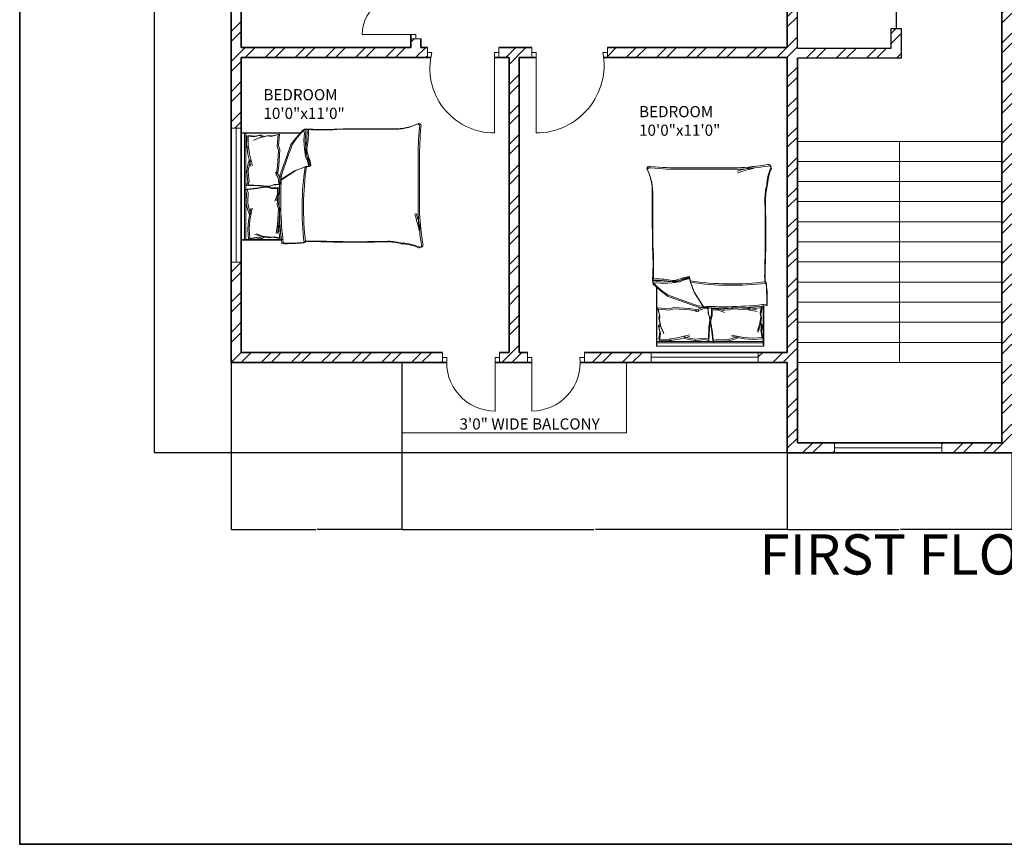
# Model space of a CAD drawing. Units: inches. Extents: x 2165 to 3042, y 1626 to 2968.
# Tile 1 of 11: x 2192 to 2633, y 1626 to 1996. Entities that reach past the tile are written whole.
import ezdxf

# ---------------------------------------------------------------- set-up
doc = ezdxf.new("R2010")
doc.units = ezdxf.units.IN
for name, color, linetype, lineweight in [('A-ANNO-DIMS', 2, 'Continuous', 18), ('A-ANNO-TEXT', 7, 'Continuous', 25), ('A-AREA-IDEN', 7, 'Continuous', 18), ('A-DOOR', 3, 'Continuous', 18), ('A-FLOR-BALC', 7, 'Continuous', 18), ('A-FLOR-EVTR', 7, 'Continuous', 25), ('A-FLOR-STRS', 7, 'Continuous', 18), ('A-FURN', 8, 'Continuous', 13), ('A-GLAZ', 4, 'Continuous', 18), ('A-WALL', 7, 'Continuous', 35), ('A-WALL-PATT', 252, 'Continuous', 13)]:
    doc.layers.add(name, color=color, linetype=linetype, lineweight=lineweight)
doc.styles.get("Standard").update_dxf_attribs({"font": 'arial.ttf'})
doc.dimstyles.get("Standard").update_dxf_attribs({"dimtxt": 0.18, "dimasz": 0.18, "dimexe": 0.18, "dimexo": 0.0625, "dimgap": 0.09, "dimtad": 0, "dimtih": 1, "dimtoh": 1, "dimdec": 4, "dimzin": 0, "dimdsep": 46, "dimtxsty": 'Standard', "dimcen": 0.09, "dimadec": 0, "dimazin": 0, "dimtfac": 1, "dimtdec": 4, "dimtofl": 0, "dimtmove": 0, "dimatfit": 3, "dimfxl": 1, "dimtolj": 1, "dimtzin": 0, "dimarcsym": 0})

# ---------------------------------------------------------------- blocks, each defined once
blk = doc.blocks.new('BED-DOUBLE')
for p, q in [((28.39, 53.1), (25.14, 49.39)), ((28.39, 53.1), (25.14, 49.39)), ((29.49, 52.95), (27.75, 52.87, 3.87)), ((29.49, 52.95), (27.75, 52.87, 3.87)), ((30.13, 53.18), (28.39, 53.1, 3.87)), ((30.13, 53.18), (28.39, 53.1, 3.87)), ((29, 51.56), (28.39, 53.1)), ((29, 51.56), (28.39, 53.1)), ((0, 51.27), (0, 51.49)), ((0, 51.49), (0.64, 51.49)), ((0, 51.27), (26.61, 51.27)), ((0, 51.27), (26.61, 51.27)), ((0, 51.27), (0, 3.48)), ((0.64, 51.49), (27.25, 51.49)), ((0.64, 51.49), (27.25, 51.49)), ((1.53, 3.48), (1.53, 51.27)), ((1.53, 3.47), (1.53, 51.27)), ((2.17, 3.7), (2.17, 51.49)), ((2.17, 3.7), (2.17, 51.49)), ((2.56, 50.11), (2.46, 44.71)), ((2.56, 50.11), (2.46, 44.71)), ((2.56, 50.11), (5.77, 49.73)), ((2.56, 50.11), (5.77, 49.73)), ((3.2, 50.34), (3.1, 44.94)), ((3.2, 50.34), (3.1, 44.94)), ((3.2, 50.34), (6.41, 49.96)), ((3.2, 50.34), (6.41, 49.96)), ((8.26, 49.31), (5.58, 48.13)), ((8.26, 49.31), (5.58, 48.13)), ((5.77, 49.73), (8.34, 50.33)), ((5.77, 49.73), (8.34, 50.33)), ((8.9, 49.54), (6.22, 48.36)), ((8.9, 49.54), (6.22, 48.36)), ((6.41, 49.96), (8.98, 50.56)), ((6.41, 49.96), (8.98, 50.56)), ((11.83, 50.11), (8.26, 49.31)), ((11.83, 50.11), (8.26, 49.31)), ((8.34, 50.33), (9.38, 49.81)), ((8.34, 50.33), (9.38, 49.81)), ((12.47, 50.34), (8.9, 49.54)), ((12.47, 50.34), (8.9, 49.54)), ((8.98, 50.56), (10.02, 50.04)), ((8.98, 50.56), (10.02, 50.04)), ((13.43, 49.92), (11.83, 50.11)), ((13.43, 49.92), (11.83, 50.11)), ((14.07, 50.15), (12.47, 50.34)), ((14.07, 50.15), (12.47, 50.34)), ((16.57, 50.7), (13.43, 49.92)), ((16.57, 50.7), (13.43, 49.92)), ((17.21, 50.93), (14.07, 50.15)), ((17.21, 50.93), (14.07, 50.15)), ((16.17, 45.57), (16.57, 50.7)), ((16.17, 45.57), (16.57, 50.7)), ((16.81, 45.79), (17.21, 50.93)), ((16.81, 45.79), (17.21, 50.93)), ((24.5, 49.16), (22.33, 46.22)), ((24.5, 49.16), (22.33, 46.22)), ((25.14, 49.39), (22.97, 46.45)), ((25.14, 49.39), (22.97, 46.45)), ((27.75, 52.87), (24.5, 49.16)), ((27.75, 52.87), (24.5, 49.16)), ((28.37, 51.33), (27.75, 52.87)), ((28.37, 51.33), (27.75, 52.87)), ((28.06, 48.23), (28.37, 51.33)), ((28.06, 48.23), (28.37, 51.33)), ((28.7, 48.46), (29, 51.56)), ((28.7, 48.46), (29, 51.56)), ((2.46, 44.71), (2.54, 45.71)), ((2.46, 44.71), (2.54, 45.71)), ((2.54, 45.71), (3.07, 41.91)), ((2.54, 45.71), (3.07, 41.91)), ((3.1, 44.94), (3.18, 45.94)), ((3.1, 44.94), (3.18, 45.94)), ((3.18, 45.94), (3.71, 42.14)), ((3.18, 45.94), (3.71, 42.14)), ((16.73, 43.61), (16.17, 45.57)), ((16.73, 43.61), (16.17, 45.57)), ((17.37, 43.83), (16.81, 45.79)), ((17.37, 43.83), (16.81, 45.79)), ((22.33, 46.22), (20.32, 40.64)), ((22.33, 46.22), (20.32, 40.64)), ((22.97, 46.45), (20.96, 40.87)), ((22.97, 46.45), (20.96, 40.87)), ((28.37, 44.36), (28.06, 48.23)), ((28.37, 44.36), (28.06, 48.23)), ((28.83, 40.95), (28.37, 44.36)), ((28.83, 40.95), (28.37, 44.36)), ((29, 44.59), (28.7, 48.46)), ((29, 44.59), (28.7, 48.46)), ((29.47, 41.18), (29, 44.59)), ((29.47, 41.18), (29, 44.59)), ((3.07, 41.91), (4.42, 36.5)), ((3.07, 41.91), (4.42, 36.49)), ((3.71, 42.14), (5.06, 36.72)), ((3.71, 42.14), (5.06, 36.72)), ((16.3, 36.6), (16.73, 43.61)), ((16.3, 36.6), (16.73, 43.61)), ((16.93, 36.82), (17.37, 43.83)), ((16.93, 36.82), (17.37, 43.83)), ((20.32, 40.64), (17.38, 32.31)), ((20.32, 40.64), (17.38, 32.31)), ((20.96, 40.87), (18.02, 32.53)), ((20.96, 40.87), (18.02, 32.53)), ((29.76, 38.94), (28.83, 40.95)), ((29.76, 38.94), (28.83, 40.95)), ((30.4, 39.17), (29.47, 41.18)), ((30.4, 39.17), (29.47, 41.18)), ((79.25, 15.06), (79.25, 39.68)), ((79.25, 15.06), (79.25, 39.68)), ((79.88, 15.29), (79.88, 39.91)), ((79.88, 15.29), (79.88, 39.91)), ((3.08, 37.14), (2.54, 34.2)), ((3.08, 37.13), (2.54, 34.2)), ((3.67, 39.2), (3.08, 37.14)), ((3.67, 39.2), (3.08, 37.13)), ((3.72, 37.36), (3.18, 34.43)), ((3.72, 37.36), (3.18, 34.43)), ((4.31, 39.43), (3.72, 37.36)), ((4.31, 39.43), (3.72, 37.36)), ((15.63, 32.56), (16.3, 36.6)), ((15.63, 32.56), (16.3, 36.6)), ((16.27, 32.79), (16.93, 36.82)), ((16.27, 32.79), (16.93, 36.82)), ((23.88, 34.45), (28.37, 36.15)), ((23.88, 34.45), (28.37, 36.15)), ((24.52, 34.68), (29, 36.38)), ((24.52, 34.68), (29, 36.38)), ((28.37, 36.15), (30.38, 36.46)), ((28.37, 36.15), (30.38, 36.46)), ((29, 36.38), (31.02, 36.69)), ((29, 36.38), (31.02, 36.69)), ((30.38, 36.46), (29.76, 38.94)), ((30.38, 36.46), (29.76, 38.94)), ((31.02, 36.69), (30.4, 39.17)), ((31.02, 36.69), (30.4, 39.17)), ((2.54, 34.2), (2.56, 33.88)), ((2.54, 34.2), (2.56, 33.88)), ((2.56, 33.88), (2.98, 29.46)), ((2.56, 33.88), (2.98, 29.46)), ((3.18, 34.43), (3.2, 34.11)), ((3.18, 34.43), (3.2, 34.11)), ((3.2, 34.11), (3.62, 29.68)), ((3.2, 34.11), (3.62, 29.68)), ((16.74, 30.75), (15.46, 33.82)), ((16.74, 30.75), (15.46, 33.82)), ((17.38, 30.98), (16.09, 34.05)), ((17.38, 30.98), (16.09, 34.05)), ((17.38, 30.26), (23.88, 34.45)), ((17.38, 30.26), (23.88, 34.45)), ((17.53, 28.53), (17.38, 30.98)), ((17.53, 28.53), (17.38, 30.98)), ((18.02, 30.49), (24.52, 34.68)), ((18.02, 30.49), (24.52, 34.68)), ((1.87, 25.98), (7.22, 26.56)), ((1.87, 25.98), (7.22, 26.56)), ((2.98, 29.46), (2.49, 27.98)), ((2.98, 29.46), (2.49, 27.98)), ((2.49, 27.98), (7.87, 27.73)), ((2.49, 27.98), (7.87, 27.73)), ((2.51, 26.21), (7.86, 26.79)), ((2.51, 26.21), (7.86, 26.79)), ((3.62, 29.68), (3.13, 28.21)), ((3.62, 29.68), (3.13, 28.21)), ((3.13, 28.21), (8.51, 27.96)), ((3.13, 28.21), (8.51, 27.96)), ((7.22, 26.56), (10.4, 27.14)), ((7.22, 26.56), (10.4, 27.14)), ((7.86, 26.79), (11.04, 27.37)), ((7.86, 26.79), (11.04, 27.37)), ((7.87, 27.73), (11.08, 27.35)), ((7.87, 27.73), (11.08, 27.35)), ((8.51, 27.96), (11.72, 27.58)), ((8.51, 27.96), (11.72, 27.58)), ((10.4, 27.14), (11.7, 27.14)), ((10.4, 27.14), (11.7, 27.14)), ((11.04, 27.37), (12.34, 27.37)), ((11.04, 27.37), (12.34, 27.37)), ((11.08, 27.35), (12.38, 27.44)), ((11.08, 27.35), (12.38, 27.44)), ((11.7, 27.14), (13.58, 26.56)), ((11.7, 27.14), (13.58, 26.56)), ((11.72, 27.58), (13.02, 27.66)), ((11.72, 27.58), (13.02, 27.66)), ((12.34, 27.37), (14.22, 26.79)), ((12.34, 27.37), (14.22, 26.79)), ((12.38, 27.44), (14.22, 28.13)), ((12.38, 27.44), (14.22, 28.13)), ((13.02, 27.66), (14.86, 28.36)), ((13.02, 27.66), (14.86, 28.36)), ((13.58, 26.56), (16.26, 26.56)), ((13.58, 26.56), (16.26, 26.56)), ((14.22, 28.13), (16.89, 28.3)), ((14.22, 28.13), (16.89, 28.3)), ((14.22, 26.79), (16.9, 26.79)), ((14.22, 26.79), (16.9, 26.79)), ((14.86, 28.36), (17.53, 28.53)), ((14.86, 28.36), (17.53, 28.53)), ((16.26, 26.56), (16.26, 24.1)), ((16.26, 26.56), (16.26, 24.1)), ((16.89, 28.3), (16.74, 30.75)), ((16.89, 28.3), (16.74, 30.75)), ((16.9, 26.79), (16.9, 24.33)), ((16.9, 26.79), (16.9, 24.33)), ((2.45, 24.54), (1.87, 25.98)), ((2.45, 24.54), (1.87, 25.98)), ((2.3, 20.09), (2.45, 24.54)), ((2.3, 20.09), (2.45, 24.54)), ((3.09, 24.77), (2.51, 26.21)), ((3.09, 24.77), (2.51, 26.21)), ((2.94, 20.32), (3.09, 24.77)), ((2.94, 20.32), (3.09, 24.77)), ((16.26, 24.1), (15.17, 20.96)), ((16.26, 24.1), (15.17, 20.96)), ((16.9, 24.33), (15.81, 21.19)), ((16.9, 24.33), (15.81, 21.19)), ((16.17, 19.38), (16.57, 24.52)), ((16.17, 19.38), (16.57, 24.52)), ((16.81, 19.61), (17.21, 24.74)), ((16.81, 19.61), (17.21, 24.74)), ((2.3, 19.77), (2.3, 20.09)), ((2.3, 19.77), (2.3, 20.09)), ((3.03, 16.88), (2.3, 19.77)), ((3.03, 16.88), (2.3, 19.77)), ((2.94, 20), (2.94, 20.32)), ((2.94, 20), (2.94, 20.32)), ((3.67, 17.11), (2.94, 20)), ((3.67, 17.11), (2.94, 20)), ((3.96, 12.34), (4.97, 17.83)), ((3.96, 12.34), (4.97, 17.83)), ((16.73, 17.42), (16.17, 19.38)), ((16.73, 17.42), (16.17, 19.38)), ((17.37, 17.65), (16.81, 19.61)), ((17.37, 17.65), (16.81, 19.61)), ((16.93, 10.64), (17.37, 17.65)), ((16.93, 10.64), (17.37, 17.65)), ((3.75, 14.85), (3.03, 16.88)), ((3.75, 14.85), (3.03, 16.88)), ((3.32, 12.11), (4.33, 17.6)), ((3.32, 12.11), (4.33, 17.6)), ((4.39, 15.08), (3.67, 17.11)), ((4.39, 15.08), (3.67, 17.11)), ((16.3, 10.41), (16.73, 17.42)), ((16.3, 10.41), (16.73, 17.42)), ((3.03, 8.28), (3.32, 12.11)), ((3.03, 8.28), (3.32, 12.11)), ((3.67, 8.51), (3.96, 12.34)), ((3.67, 8.51), (3.96, 12.34)), ((15.63, 6.38), (16.3, 10.41)), ((15.63, 6.38), (16.3, 10.41)), ((16.27, 6.61), (16.93, 10.64)), ((16.27, 6.61), (16.93, 10.64)), ((16.3, 10.41), (16.62, 9.28)), ((16.3, 10.41), (16.62, 9.28)), ((16.62, 9.28), (17.34, 4.18)), ((16.62, 9.28), (17.34, 4.18)), ((16.93, 10.64), (17.26, 9.51)), ((16.93, 10.64), (17.26, 9.51)), ((17.26, 9.51), (17.98, 4.41)), ((17.26, 9.51), (17.98, 4.41)), ((3.01, 8.18), (3.03, 8.28)), ((3.01, 8.18), (3.03, 8.28)), ((3.34, 3.9), (3.01, 8.18)), ((3.34, 3.9), (3.01, 8.18)), ((3.32, 3.89), (6.5, 4.47)), ((3.32, 3.89), (6.5, 4.47)), ((3.65, 8.41), (3.67, 8.51)), ((3.65, 8.41), (3.67, 8.51)), ((3.98, 4.13), (3.65, 8.41)), ((3.98, 4.13), (3.65, 8.41)), ((3.96, 4.12), (7.14, 4.7)), ((3.96, 4.12), (7.14, 4.7)), ((8.96, 5.05), (6.21, 6.06)), ((8.96, 5.05), (6.21, 6.06)), ((6.5, 4.47), (9.1, 4.04)), ((6.5, 4.47), (9.1, 4.04)), ((9.59, 5.28), (6.85, 6.29)), ((9.59, 5.28), (6.85, 6.29)), ((7.14, 4.7), (9.74, 4.27)), ((7.14, 4.7), (9.74, 4.27)), ((12.57, 4.47), (8.96, 5.05)), ((12.57, 4.47), (8.96, 5.05)), ((9.1, 4.04), (10.11, 4.62)), ((9.1, 4.04), (10.11, 4.62)), ((13.21, 4.7), (9.59, 5.28)), ((13.21, 4.7), (9.59, 5.28)), ((9.74, 4.27), (10.75, 4.85)), ((9.74, 4.27), (10.75, 4.85)), ((14.16, 4.76), (12.57, 4.47)), ((14.16, 4.76), (12.57, 4.47)), ((14.8, 4.99), (13.21, 4.7)), ((14.8, 4.99), (13.21, 4.7)), ((17.34, 4.18), (14.16, 4.76)), ((17.34, 4.18), (14.16, 4.76)), ((17.98, 4.41), (14.8, 4.99)), ((17.98, 4.41), (14.8, 4.99)), ((18.11, 3.48), (0, 3.48)), ((18.11, 3.47), (0, 3.47)), ((18.75, 3.7), (0.64, 3.7)), ((18.75, 3.7), (0.64, 3.7))]:
    blk.add_line(p, q)
for centre, radius, start, end in [((-6.66, 51.33), 36.18, 349.8763, 2.5657), ((-6.66, 51.33), 36.18, 349.8763, 2.5657), ((36.32, 182.27), 129.5, 266.9791, 273.8365), ((36.32, 182.27), 129.5, 266.9791, 273.8365), ((-6.02, 51.56), 36.18, 349.8763, 2.5657), ((-6.02, 51.56), 36.18, 349.8763, 2.5657), ((36.95, 182.49), 129.5, 266.9791, 273.8365), ((36.95, 182.49), 129.5, 266.9791, 273.8365), ((67.82, -4508.74), 4561.86, 90.00217, 90.28689), ((67.82, -4508.74), 4561.86, 90.00217, 90.28689), ((68.46, -4508.52), 4561.86, 90.00217, 90.28689), ((68.46, -4508.52), 4561.86, 90.00217, 90.28689), ((68.67, 76.16), 23.07, 267.4714, 296.4681), ((68.67, 76.16), 23.07, 267.4714, 296.4681), ((69.31, 76.39), 23.07, 267.4714, 296.4681), ((69.31, 76.39), 23.07, 267.4714, 296.4681), ((78.87, 54.41), 1.1, 332.6588, 86.02), ((78.87, 54.41), 1.1, 332.6588, 86.02), ((212.28, 41.15), 133.04, 174.4998, 180.6351), ((212.28, 41.15), 133.04, 174.4998, 180.6351), ((79.51, 54.64), 1.1, 332.6588, 86.02), ((79.51, 54.64), 1.1, 332.6588, 86.02), ((212.92, 41.38), 133.04, 174.4998, 180.6351), ((212.92, 41.38), 133.04, 174.4998, 180.6351), ((35.07, 43.74), 6.22, 168.6608, 203.7384), ((35.07, 43.74), 6.22, 168.6608, 203.7384), ((35.71, 43.97), 6.22, 168.6608, 203.7384), ((35.71, 43.97), 6.22, 168.6608, 203.7384), ((1.48, 31.15), 29.65, 10.6617, 19.8806), ((1.48, 31.15), 29.65, 10.6617, 19.8806), ((2.12, 31.38), 29.65, 10.6617, 19.8806), ((2.12, 31.38), 29.65, 10.6617, 19.8806), ((156.32, 17.76), 129.02, 171.7845, 186.9006), ((156.32, 17.76), 129.02, 171.7845, 186.9006), ((156.96, 17.98), 129.02, 171.7845, 186.9006), ((156.96, 17.98), 129.02, 171.7845, 186.9006), ((30.44, 36.64), 0.185, 250.2464, 1.1377), ((30.44, 36.64), 0.185, 250.2464, 1.1377), ((31.08, 36.86), 0.185, 250.2464, 1.1377), ((31.08, 36.86), 0.185, 250.2464, 1.1377), ((182.05, 21.36), 164.97, 176.0865, 186.7821), ((182.05, 21.36), 164.97, 176.0865, 186.7821), ((182.69, 21.59), 164.97, 176.0865, 186.7821), ((182.69, 21.59), 164.97, 176.0865, 186.7821), ((-23.71, -17.22), 106.46, 13.3832, 17.7053), ((-23.71, -17.22), 106.46, 13.3832, 17.7053), ((-23.07, -16.99), 106.46, 13.3832, 17.7053), ((-23.07, -16.99), 106.46, 13.3832, 17.7053), ((200.84, 21.43), 121.76, 182.9958, 189.4091), ((200.84, 21.43), 121.76, 182.9958, 189.4091), ((201.48, 21.66), 121.76, 182.9958, 189.4091), ((201.48, 21.65), 121.76, 182.9958, 189.4091), ((20.1, 85.16), 83.31, 268.7218, 275.604), ((20.1, 85.16), 83.31, 268.7218, 275.604), ((20.74, 85.39), 83.31, 268.7218, 275.604), ((20.74, 85.39), 83.31, 268.7218, 275.604), ((31.17, -167.31), 170.11, 88.4762, 91.0082), ((31.17, -167.31), 170.11, 88.4762, 91.0082), ((31.81, -167.08), 170.11, 88.4762, 91.0082), ((31.81, -167.08), 170.11, 88.4762, 91.0082), ((50.61, 484.82), 482.31, 268.2277, 271.7185), ((50.61, 484.82), 482.31, 268.2277, 271.7185), ((51.25, 485.05), 482.31, 268.2277, 271.7185), ((51.25, 485.05), 482.31, 268.2277, 271.7185), ((64.52, -26.9), 29.63, 76.0648, 88.9113), ((64.52, -26.9), 29.63, 76.0648, 88.9113), ((65.15, -26.67), 29.63, 76.0648, 88.9113), ((65.15, -26.67), 29.63, 76.0648, 88.9113), ((70.28, -21.66), 23.56, 67.9751, 86.652), ((70.28, -21.66), 23.56, 67.9751, 86.652), ((70.92, -21.43), 23.56, 67.9751, 86.652), ((70.92, -21.43), 23.56, 67.9751, 86.652), ((79.72, 1.09), 1.09, 236.1736, 23.4781), ((79.72, 1.09), 1.09, 236.1736, 23.4781), ((80.36, 1.32), 1.09, 236.1736, 23.4781), ((80.36, 1.32), 1.09, 236.1736, 23.4781)]:
    blk.add_arc(centre, radius, start, end)
blk = doc.blocks.new('BALCONY-RAIL-PLAN')
for p, q in [((0, 31.5), (0, 0)), ((100.5, 31.5), (100.5, 0)), ((100.5, 0), (0, 0))]:
    blk.add_line(p, q)
blk = doc.blocks.new('WIN-60-B')
for p, q in [((0, 4.5), (0, 0)), ((60, 2.25), (60, 4.5)), ((60, 4.5), (60, 0)), ((0, 0), (0, 2.25)), ((0, 2.25), (60, 2.25))]:
    blk.add_line(p, q)
blk = doc.blocks.new('WIN-48')
for p, q in [((0, 4.5), (0, 0)), ((48, 2.25), (48, 4.5)), ((48, 4.5), (48, 0)), ((0, 0), (0, 2.25)), ((0, 2.25), (48, 2.25))]:
    blk.add_line(p, q)
blk = doc.blocks.new('*D51')
at = {"layer": 'A-ANNO-DIMS', "color": 0, "lineweight": -2, "transparency": 16777216}
for p, q in [((2387.04, 2363.58), (2252.12, 2363.58)), ((2252.3, 2363.4), (2252.3, 2082.76)), ((2252.3, 1801.76), (2252.3, 2082.4)), ((2535.54, 1801.58), (2252.12, 1801.58))]:
    blk.add_line(p, q, dxfattribs=at)
at = {"layer": 'A-ANNO-DIMS', "color": 0, "transparency": 16777216}
for points in [[(2252.27, 2363.4), (2252.33, 2363.4), (2252.3, 2363.58)], [(2252.27, 1801.76), (2252.33, 1801.76), (2252.3, 1801.58)]]:
    blk.add_solid(points, dxfattribs=at)
at = {"layer": 'Defpoints', "color": 0, "transparency": 16777216}
for p in [(2252.3, 2363.58), (2387.1, 2363.58), (2535.6, 1801.58)]:
    blk.add_point(p, dxfattribs=at)
at = {"layer": 'A-ANNO-DIMS', "color": 0, "transparency": 16777216, "insert": (2252.3, 2082.58), "char_height": 0.18, "attachment_point": 5}
blk.add_mtext('\\A1;562', dxfattribs=at)
blk = doc.blocks.new('*D52')
at = {"layer": 'A-ANNO-DIMS', "color": 0, "lineweight": -2, "transparency": 16777216}
for p, q in [((2286.6, 1842.02), (2286.6, 1767.1)), ((2363.1, 1842.02), (2363.1, 1767.1)), ((2286.78, 1767.28), (2324.53, 1767.28)), ((2362.92, 1767.28), (2325.18, 1767.28))]:
    blk.add_line(p, q, dxfattribs=at)
at = {"layer": 'A-ANNO-DIMS', "color": 0, "transparency": 16777216}
for points in [[(2286.78, 1767.31), (2286.78, 1767.25), (2286.6, 1767.28)], [(2362.92, 1767.31), (2362.92, 1767.25), (2363.1, 1767.28)]]:
    blk.add_solid(points, dxfattribs=at)
at = {"layer": 'Defpoints', "color": 0, "transparency": 16777216}
for p in [(2286.6, 1842.08), (2363.1, 1842.08), (2363.1, 1767.28)]:
    blk.add_point(p, dxfattribs=at)
at = {"layer": 'A-ANNO-DIMS', "color": 0, "transparency": 16777216, "insert": (2324.85, 1767.28), "char_height": 0.18, "attachment_point": 5}
blk.add_mtext('\\A1;76.5', dxfattribs=at)
blk = doc.blocks.new('*D53')
at = {"layer": 'A-ANNO-DIMS', "color": 0, "lineweight": -2, "transparency": 16777216}
for p, q in [((2363.1, 1842.02), (2363.1, 1767.1)), ((2535.6, 1842.02), (2535.6, 1767.1)), ((2363.28, 1767.28), (2448.97, 1767.28)), ((2535.42, 1767.28), (2449.74, 1767.28))]:
    blk.add_line(p, q, dxfattribs=at)
at = {"layer": 'A-ANNO-DIMS', "color": 0, "transparency": 16777216}
for points in [[(2363.28, 1767.31), (2363.28, 1767.25), (2363.1, 1767.28)], [(2535.42, 1767.31), (2535.42, 1767.25), (2535.6, 1767.28)]]:
    blk.add_solid(points, dxfattribs=at)
at = {"layer": 'Defpoints', "color": 0, "transparency": 16777216}
for p in [(2363.1, 1842.08), (2535.6, 1842.08), (2535.6, 1767.28)]:
    blk.add_point(p, dxfattribs=at)
at = {"layer": 'A-ANNO-DIMS', "color": 0, "transparency": 16777216, "insert": (2449.35, 1767.28), "char_height": 0.18, "attachment_point": 5}
blk.add_mtext('\\A1;172.5', dxfattribs=at)
blk = doc.blocks.new('*D54')
at = {"layer": 'A-ANNO-DIMS', "color": 0, "lineweight": -2, "transparency": 16777216}
for p, q in [((2535.6, 1801.52), (2535.6, 1767.1)), ((2636.1, 1801.52), (2636.1, 1767.1)), ((2535.78, 1767.28), (2585.47, 1767.28)), ((2635.92, 1767.28), (2586.24, 1767.28))]:
    blk.add_line(p, q, dxfattribs=at)
at = {"layer": 'A-ANNO-DIMS', "color": 0, "transparency": 16777216}
for points in [[(2535.78, 1767.31), (2535.78, 1767.25), (2535.6, 1767.28)], [(2635.92, 1767.31), (2635.92, 1767.25), (2636.1, 1767.28)]]:
    blk.add_solid(points, dxfattribs=at)
at = {"layer": 'Defpoints', "color": 0, "transparency": 16777216}
for p in [(2535.6, 1801.58), (2636.1, 1801.58), (2636.1, 1767.28)]:
    blk.add_point(p, dxfattribs=at)
at = {"layer": 'A-ANNO-DIMS', "color": 0, "transparency": 16777216, "insert": (2585.85, 1767.28), "char_height": 0.18, "attachment_point": 5}
blk.add_mtext('\\A1;100.5', dxfattribs=at)

msp = doc.modelspace()

# ---------------------------------------------------------------- hatches: boundary and pattern name
at = {"layer": 'A-WALL-PATT'}
h = msp.add_hatch(dxfattribs=at)
h.set_pattern_fill('ANSI32', color=256)
h.paths.add_polyline_path([(2406.4931, 2332.0783), (2286.6045, 2332.0783), (2286.6045, 2310.967), (2288.8545, 2310.967), (2291.1045, 2310.967), (2291.1045, 2327.5783), (2406.4931, 2327.5783), (2406.4931, 2329.8283)])
h.paths.add_polyline_path([(2439.6045, 2327.5783), (2444.9584, 2327.5783), (2444.9584, 2332.0783), (2430.2901, 2332.0783), (2430.2901, 2329.8283), (2430.2901, 2327.5783), (2435.1045, 2327.5783), (2435.1045, 2219.5783), (2431.0902, 2219.5783), (2431.0902, 2215.0783), (2435.1045, 2215.0783), (2444.1108, 2215.0783), (2444.1108, 2217.3283), (2444.1108, 2219.5783), (2439.6045, 2219.5783)])
h.paths.add_polyline_path([(2497.5418, 2329.8283), (2497.5418, 2332.0783), (2470.1978, 2332.0783), (2470.1978, 2327.5783), (2497.5418, 2327.5783)])
h.paths.add_polyline_path([(2617.9543, 2332.0783), (2557.5418, 2332.0783), (2557.5418, 2327.5783), (2583.6045, 2327.5783), (2583.6045, 2219.5783), (2474.0523, 2219.5783), (2474.0523, 2215.0783), (2583.6045, 2215.0783), (2583.6045, 2107.0783), (2579.3609, 2107.0783), (2579.3609, 2102.5783), (2588.1045, 2102.5783), (2593.5283, 2102.5783), (2593.5283, 2104.8283), (2593.5283, 2107.0783), (2588.1045, 2107.0783), (2588.1045, 2215.0783), (2691.2325, 2215.0783), (2691.2325, 2217.3283), (2691.2325, 2219.5783), (2588.1045, 2219.5783), (2588.1045, 2327.5783), (2617.9543, 2327.5783)])
h.paths.add_polyline_path([(2702.4444, 2329.8283), (2702.4444, 2332.0783), (2677.9543, 2332.0783), (2677.9543, 2327.5783), (2702.4444, 2327.5783)])
h.paths.add_polyline_path([(2736.6045, 2327.5783), (2742.5161, 2327.5783), (2742.5161, 2329.8283), (2742.5161, 2332.0783), (2727.7639, 2332.0783), (2727.7639, 2329.8283), (2727.7639, 2327.5783), (2732.1045, 2327.5783), (2732.1045, 2219.5783), (2726.4404, 2219.5783), (2726.4404, 2215.0783), (2732.1045, 2215.0783), (2742.7291, 2215.0783), (2742.7291, 2217.3283), (2742.7291, 2219.5783), (2736.6045, 2219.5783)])
h.paths.add_polyline_path([(2885.1045, 2332.0783), (2768.4887, 2332.0783), (2768.4887, 2327.5783), (2784.6045, 2327.5783), (2880.6045, 2327.5783), (2880.6045, 2310.967), (2885.1045, 2310.967)])
h.paths.add_polyline_path([(2885.1045, 2250.967), (2880.6045, 2250.967), (2880.6045, 2219.5783), (2776.5755, 2219.5783), (2776.5755, 2215.0783), (2788.1045, 2215.0783), (2788.1045, 2209.8634), (2790.3545, 2209.8634), (2792.6045, 2209.8634), (2792.6045, 2215.0783), (2880.6045, 2215.0783), (2880.6045, 2139.0783), (2871.2037, 2139.0783), (2871.2037, 2134.5783), (2885.1045, 2134.5783)])
h.paths.add_polyline_path([(2545.013, 2107.0783), (2474.0523, 2107.0783), (2291.1045, 2107.0783), (2291.1045, 2102.5783), (2535.6045, 2102.5783), (2535.6045, 2096.8046), (2537.8545, 2096.8046), (2540.1045, 2096.8046), (2540.1045, 2102.5783), (2545.013, 2102.5783), (2545.013, 2104.8283)])
h.paths.add_polyline_path([(2397.7297, 2217.3283), (2397.7297, 2219.5783), (2291.1045, 2219.5783), (2291.1045, 2250.967), (2286.6045, 2250.967), (2286.6045, 2206.1346), (2288.8545, 2206.1346), (2291.1045, 2206.1346), (2291.1045, 2215.0783), (2367.1045, 2215.0783), (2367.1045, 2212.2868), (2371.6045, 2212.2868), (2371.6045, 2215.0783), (2397.7297, 2215.0783)])
h.paths.add_polyline_path([(2291.1045, 1978.5783), (2367.1045, 1978.5783), (2371.6045, 1978.5783), (2373.2641, 1978.5783), (2374.4883, 1978.5783), (2374.4883, 1980.8283), (2374.4883, 1983.0783), (2371.6045, 1983.0783), (2371.6045, 1986.964), (2369.9051, 1986.964), (2369.3545, 1986.964), (2367.1045, 1986.964), (2367.1045, 1983.0783), (2291.1045, 1983.0783), (2291.1045, 2001.1808), (2286.6045, 2001.1808), (2286.6045, 1947.0203), (2288.8545, 1947.0203), (2291.1045, 1947.0203)])
h.paths.add_polyline_path([(2291.1045, 1887.0203), (2286.6045, 1887.0203), (2286.6045, 1842.0783), (2381.2561, 1842.0783), (2381.2561, 1844.3283), (2381.2561, 1846.5783), (2363.1045, 1846.5783), (2291.1045, 1846.5783)])
h.paths.add_polyline_path([(2415.6045, 1978.5783), (2421.1681, 1978.5783), (2421.1681, 1983.0783), (2415.6045, 1983.0783), (2406.5227, 1983.0783), (2406.5227, 1980.8283), (2406.5227, 1978.5783), (2411.1045, 1978.5783), (2411.1045, 1846.5783), (2406.7549, 1846.5783), (2406.7549, 1842.0783), (2419.2885, 1842.0783), (2419.2885, 1844.3283), (2419.2885, 1846.5783), (2415.6045, 1846.5783)])
h.paths.add_polyline_path([(2586.6045, 1982.779), (2586.6045, 1991.5911), (2582.1045, 1991.5911), (2582.1045, 1982.779), (2540.1045, 1982.779), (2540.1045, 2036.779), (2582.1045, 2036.779), (2582.1045, 2027.6051), (2586.6045, 2027.6051), (2586.6045, 2041.279), (2582.1045, 2041.279), (2540.1045, 2041.279), (2540.1045, 2063.9064), (2537.8545, 2063.9064), (2535.6045, 2063.9064), (2535.6045, 1983.0783), (2455.068, 1983.0783), (2455.068, 1978.5783), (2535.6045, 1978.5783), (2535.6045, 1846.5783), (2522.622, 1846.5783), (2522.622, 1842.0783), (2535.6045, 1842.0783), (2535.6045, 1806.0783), (2535.6045, 1801.5783), (2556.726, 1801.5783), (2556.726, 1803.8283), (2556.726, 1806.0783), (2540.1045, 1806.0783), (2540.1045, 1842.0783), (2540.1045, 1846.5783), (2540.1045, 1978.279), (2586.6045, 1978.279)])
h.paths.add_polyline_path([(2636.1045, 1978.5783), (2717.6642, 1978.5783), (2717.6642, 1980.8283), (2717.6642, 1983.0783), (2636.1045, 1983.0783), (2636.1045, 2063.9064), (2633.8545, 2063.9064), (2631.6045, 2063.9064), (2631.6045, 1846.5783), (2631.6045, 1842.0783), (2631.6045, 1806.0783), (2604.726, 1806.0783), (2604.726, 1801.5783), (2636.1045, 1801.5783), (2636.1045, 1842.0783), (2644.3411, 1842.0783), (2644.3411, 1844.3283), (2644.3411, 1846.5783), (2636.1045, 1846.5783)])
h.paths.add_polyline_path([(2760.6045, 1978.5783), (2764.9931, 1978.5783), (2764.9931, 1983.0783), (2750.4727, 1983.0783), (2750.4727, 1980.8283), (2750.4727, 1978.5783), (2756.1045, 1978.5783), (2756.1045, 1846.5783), (2749.4543, 1846.5783), (2749.4543, 1842.0783), (2765.1894, 1842.0783), (2765.1894, 1846.5783), (2760.6045, 1846.5783)])
h.paths.add_polyline_path([(2880.6045, 1983.0783), (2804.6045, 1983.0783), (2804.6045, 1988.3825), (2802.3545, 1988.3825), (2800.1045, 1988.3825), (2800.1045, 1983.0783), (2800.1045, 1978.5783), (2880.6045, 1978.5783)])
h.paths.add_polyline_path([(2885.1045, 2075.5783), (2871.2037, 2075.5783), (2871.2037, 2071.0783), (2880.6045, 2071.0783), (2880.6045, 1948.8144), (2885.1045, 1948.8144)])
h.paths.add_polyline_path([(2885.1045, 1888.8144), (2880.6045, 1888.8144), (2880.6045, 1846.5783), (2792.1167, 1846.5783), (2792.1167, 1842.0783), (2885.1045, 1842.0783)])
h.paths.add_polyline_path([(2724.4848, 1846.5783), (2708.1045, 1846.5783), (2692.3411, 1846.5783), (2692.3411, 1842.0783), (2724.4848, 1842.0783), (2724.4848, 1844.3283)])
h.paths.add_polyline_path([(2474.622, 1844.4672), (2474.622, 1846.5783), (2444.7417, 1846.5783), (2444.7417, 1842.0783), (2474.622, 1842.0783)])

# ---------------------------------------------------------------- linework, layer by layer
at = {"layer": 'A-DOOR'}
for p, q in [((2369.3545, 1988.964), (2345.3545, 1988.964)), ((2369.3545, 1986.964), (2369.3545, 1988.964)), ((2367.1045, 1986.964), (2371.6045, 1986.964)), ((2369.9051, 1986.964), (2369.3545, 1986.964)), ((2371.6045, 1986.964), (2369.9051, 1986.964)), ((2374.4883, 1983.0783), (2374.4883, 1978.5783)), ((2374.4883, 1978.5783), (2374.4883, 1980.8283)), ((2374.4883, 1980.8283), (2376.4883, 1980.8283)), ((2406.5227, 1980.8283), (2404.5227, 1980.8283)), ((2404.5227, 1980.8283), (2404.5227, 1944.8283)), ((2406.5227, 1978.5783), (2406.5227, 1983.0783)), ((2406.5227, 1983.0783), (2406.5227, 1980.8283)), ((2421.1681, 1978.5783), (2421.1681, 1983.0783)), ((2421.1681, 1983.0783), (2421.1681, 1980.8283)), ((2421.1681, 1980.8283), (2421.1681, 1980.8283)), ((2421.1681, 1980.8283), (2423.1681, 1980.8283)), ((2423.1681, 1980.8283), (2423.1681, 1944.8283)), ((2455.068, 1980.8283), (2453.068, 1980.8283)), ((2455.068, 1983.0783), (2455.068, 1978.5783)), ((2455.068, 1978.5783), (2455.068, 1980.8283)), ((2381.2561, 1846.5783), (2381.2561, 1842.0783)), ((2381.2561, 1842.0783), (2381.2561, 1844.3283)), ((2381.2561, 1844.3283), (2383.2561, 1844.3283)), ((2406.7549, 1844.3283), (2404.7549, 1844.3283)), ((2404.7549, 1844.3283), (2404.7549, 1820.3283)), ((2406.7549, 1846.5783), (2406.7549, 1842.0783)), ((2406.7549, 1842.0783), (2406.7549, 1844.3283)), ((2419.2885, 1846.5783), (2419.2885, 1842.0783)), ((2419.2885, 1842.0783), (2419.2885, 1844.3283)), ((2419.2885, 1844.3283), (2421.2885, 1844.3283)), ((2421.2885, 1844.3283), (2421.2885, 1820.3283)), ((2444.7417, 1844.3283), (2442.7417, 1844.3283)), ((2444.7417, 1846.5783), (2444.7417, 1842.0783)), ((2444.7417, 1842.0783), (2444.7417, 1844.3283))]:
    msp.add_line(p, q, dxfattribs=at)
for centre, radius, start, end in [((2362.5919, 1988.964), 17.2375, 66.901381, 180), ((2404.5227, 1973.744), 28.9157, 165.818174, 270), ((2423.1681, 1975.245), 30.4167, 270, 10.577168), ((2404.7549, 1841.9575), 21.6291, 173.706943, 270), ((2421.2885, 1841.9166), 21.5883, 270, 6.414023)]:
    msp.add_arc(centre, radius, start, end, dxfattribs=at)
at = {"layer": 'A-FLOR-EVTR'}
for p, q in [((2540.1045, 1982.779), (2540.1045, 2036.779)), ((2584.3545, 2027.6051), (2584.3545, 1991.5911)), ((2582.1045, 1982.779), (2582.1045, 1991.5911)), ((2582.1045, 1991.5911), (2586.6045, 1991.5911)), ((2586.6045, 1991.5911), (2586.6045, 1982.779)), ((2540.1045, 1982.779), (2582.1045, 1982.779)), ((2586.6045, 1982.779), (2586.6045, 1978.279)), ((2586.6045, 1978.279), (2540.1045, 1978.279))]:
    msp.add_line(p, q, dxfattribs=at)
at = {"layer": 'A-FLOR-STRS'}
for p, q in [((2540.1045, 1941.0783), (2631.6045, 1941.0783)), ((2585.8545, 1842.0783), (2585.8545, 1941.0783)), ((2540.1045, 1932.0783), (2631.6045, 1932.0783)), ((2540.1045, 1923.0783), (2631.6045, 1923.0783)), ((2540.1045, 1914.0783), (2631.6045, 1914.0783)), ((2540.1045, 1905.0783), (2631.6045, 1905.0783)), ((2540.1045, 1896.0783), (2631.6045, 1896.0783)), ((2540.1045, 1887.0783), (2631.6045, 1887.0783)), ((2540.1045, 1878.0783), (2631.6045, 1878.0783)), ((2540.1045, 1869.0783), (2631.6045, 1869.0783)), ((2540.1045, 1860.0783), (2631.6045, 1860.0783)), ((2540.1045, 1851.0783), (2631.6045, 1851.0783)), ((2540.1045, 1842.0783), (2631.6045, 1842.0783))]:
    msp.add_line(p, q, dxfattribs=at)
at = {"layer": 'A-GLAZ'}
for p, q in [((2474.622, 1846.5783), (2474.622, 1843.4821)), ((2474.622, 1842.0783), (2474.622, 1844.4672)), ((2474.622, 1844.4672), (2522.622, 1844.4672)), ((2474.622, 1843.4821), (2474.622, 1842.0783)), ((2522.622, 1844.4672), (2522.622, 1846.5783)), ((2522.622, 1846.5783), (2522.622, 1842.0783))]:
    msp.add_line(p, q, dxfattribs=at)
at = {"layer": 'A-WALL'}
for p, q in [((2286.6045, 2332.0783), (2286.6045, 1842.0783)), ((2535.6045, 1983.0783), (2535.6045, 2065.4985)), ((2631.6045, 2063.9064), (2631.6045, 1846.5783)), ((2291.1045, 2038.0783), (2291.1045, 1983.0783)), ((2367.1045, 1988.964), (2367.1045, 1983.0783)), ((2371.6045, 1983.0783), (2371.6045, 1986.964)), ((2367.1045, 1983.0783), (2291.1045, 1983.0783)), ((2374.4883, 1983.0783), (2371.6045, 1983.0783)), ((2415.6045, 1983.0783), (2406.5227, 1983.0783)), ((2415.6045, 1983.0783), (2421.1681, 1983.0783)), ((2455.068, 1983.0783), (2535.6045, 1983.0783)), ((2291.1045, 1978.5783), (2367.1045, 1978.5783)), ((2291.1045, 1978.5783), (2291.1045, 1846.5783)), ((2291.1045, 1978.5783), (2291.1045, 1846.5783)), ((2367.1045, 1978.5783), (2371.6045, 1978.5783)), ((2371.6045, 1978.5783), (2373.2641, 1978.5783)), ((2373.2641, 1978.5783), (2376.014, 1978.5783)), ((2404.5227, 1978.5783), (2411.1045, 1978.5783)), ((2411.1045, 1846.5783), (2411.1045, 1978.5783)), ((2411.1045, 1978.5783), (2411.1045, 1978.5783)), ((2415.6045, 1846.5783), (2415.6045, 1978.5783)), ((2415.6045, 1978.5783), (2423.1681, 1978.5783)), ((2453.4016, 1978.5783), (2535.6045, 1978.5783)), ((2535.6045, 1846.5783), (2535.6045, 1978.5783)), ((2540.1045, 1846.5783), (2540.1045, 1978.279)), ((2291.1045, 1846.5783), (2381.2561, 1846.5783)), ((2381.2561, 1846.5783), (2363.1045, 1846.5783)), ((2411.1045, 1846.5783), (2406.7549, 1846.5783)), ((2406.7549, 1846.5783), (2411.1045, 1846.5783)), ((2415.6045, 1846.5783), (2419.2885, 1846.5783)), ((2415.6045, 1846.5783), (2419.2885, 1846.5783)), ((2444.7417, 1846.5783), (2535.6045, 1846.5783)), ((2444.7417, 1846.5783), (2463.6045, 1846.5783)), ((2540.1045, 1846.5783), (2540.1045, 1842.0783)), ((2631.6045, 1842.0783), (2631.6045, 1846.5783)), ((2286.6045, 1842.0783), (2383.1261, 1842.0783)), ((2404.7549, 1842.0783), (2421.2885, 1842.0783)), ((2411.1045, 1842.0783), (2415.6045, 1842.0783)), ((2442.8762, 1842.0783), (2535.6045, 1842.0783)), ((2535.6045, 1842.0783), (2535.6045, 1806.0783)), ((2540.1045, 1842.0783), (2540.1045, 1806.0783)), ((2631.6045, 1806.0783), (2631.6045, 1842.0783)), ((2535.6045, 1806.0783), (2535.6045, 1801.5783)), ((2540.1045, 1806.0783), (2631.6045, 1806.0783)), ((2535.6045, 1801.5783), (2636.1045, 1801.5783))]:
    msp.add_line(p, q, dxfattribs=at)
msp.add_lwpolyline([(2191.9961, 2967.8547), (3042.3708, 2967.8547), (3042.3708, 1626.3264), (2191.9961, 1626.3264)], close=True, dxfattribs=at)

# ---------------------------------------------------------------- block references
at = {"layer": 'A-FLOR-BALC'}
msp.add_blockref('BALCONY-RAIL-PLAN', (2363.104, 1810.578), dxfattribs=at)
at = {"layer": 'A-FURN'}
msp.add_blockref('BED-DOUBLE', (2291.104, 1893.4053), dxfattribs=at)
at = {"layer": 'A-FURN', "rotation": 89.99999983324265}
msp.add_blockref('BED-DOUBLE', (2528.4904, 1849.3206), dxfattribs=at)
at = {"layer": 'A-GLAZ'}
for name, p, rotation in [('WIN-60-B', (2286.6041, 1947.0201), 270), ('WIN-48', (2604.7261, 1806.0786), 180)]:
    msp.add_blockref(name, p, dxfattribs=dict(at, rotation=rotation))

# ---------------------------------------------------------------- texts
at = {"layer": 'A-ANNO-TEXT', "insert": (2523.1237, 1765.1301), "char_height": 18, "attachment_point": 1}
msp.add_mtext_dynamic_manual_height_columns('FIRST FLOOR PLAN', width=534.683278, gutter_width=12.5, heights=[0], dxfattribs=at)
at = {"layer": 'A-AREA-IDEN', "char_height": 5, "attachment_point": 1}
for s, width, insert in [('BEDROOM\\P10\'0"x11\'0"', 127.172024, (2301.1123, 1964.4597)), ('BEDROOM\\P10\'0"x11\'0"', 105.623691, (2469.2407, 1956.8959)), ('3\'0" WIDE BALCONY', 69.420923, (2388.8796, 1817.0342))]:
    msp.add_mtext_dynamic_manual_height_columns(s, width=width, gutter_width=12.5, heights=[0], dxfattribs=dict(at, insert=insert))

# ---------------------------------------------------------------- dimensions: what is measured, and where the dimension line sits
at = {"layer": 'A-ANNO-DIMS'}
dim = msp.add_linear_dim(base=(2252.3045, 2363.5783), p1=(2535.6045, 1801.5783), p2=(2387.1045, 2363.5783), angle=90, dimstyle='Standard', override={"dimdec": 0, "dimlfac": 1, "dimrnd": 0, "dimzin": 0, "dimdsep": 46, "dimlunit": 2}, dxfattribs=at)
dim.commit()
dim.dimension.update_dxf_attribs({"geometry": '*D51', "text_midpoint": (2252.3045, 2082.5783)})
for base, p1, p2, picture, middle in [((2363.1045, 1767.2783), (2286.6045, 1842.0783), (2363.1045, 1842.0783), '*D52', (2324.8545, 1767.2783)), ((2535.6045, 1767.2783), (2363.1045, 1842.0783), (2535.6045, 1842.0783), '*D53', (2449.3545, 1767.2783)), ((2636.1045, 1767.2783), (2535.6045, 1801.5783), (2636.1045, 1801.5783), '*D54', (2585.8545, 1767.2783))]:
    dim = msp.add_linear_dim(base=base, p1=p1, p2=p2, dimstyle='Standard', override={"dimdec": 1, "dimlfac": 1, "dimrnd": 0, "dimzin": 0, "dimdsep": 46, "dimlunit": 2}, dxfattribs=at)
    dim.commit()
    dim.dimension.update_dxf_attribs({"geometry": picture, "text_midpoint": middle})

doc.saveas('drawing.dxf')
